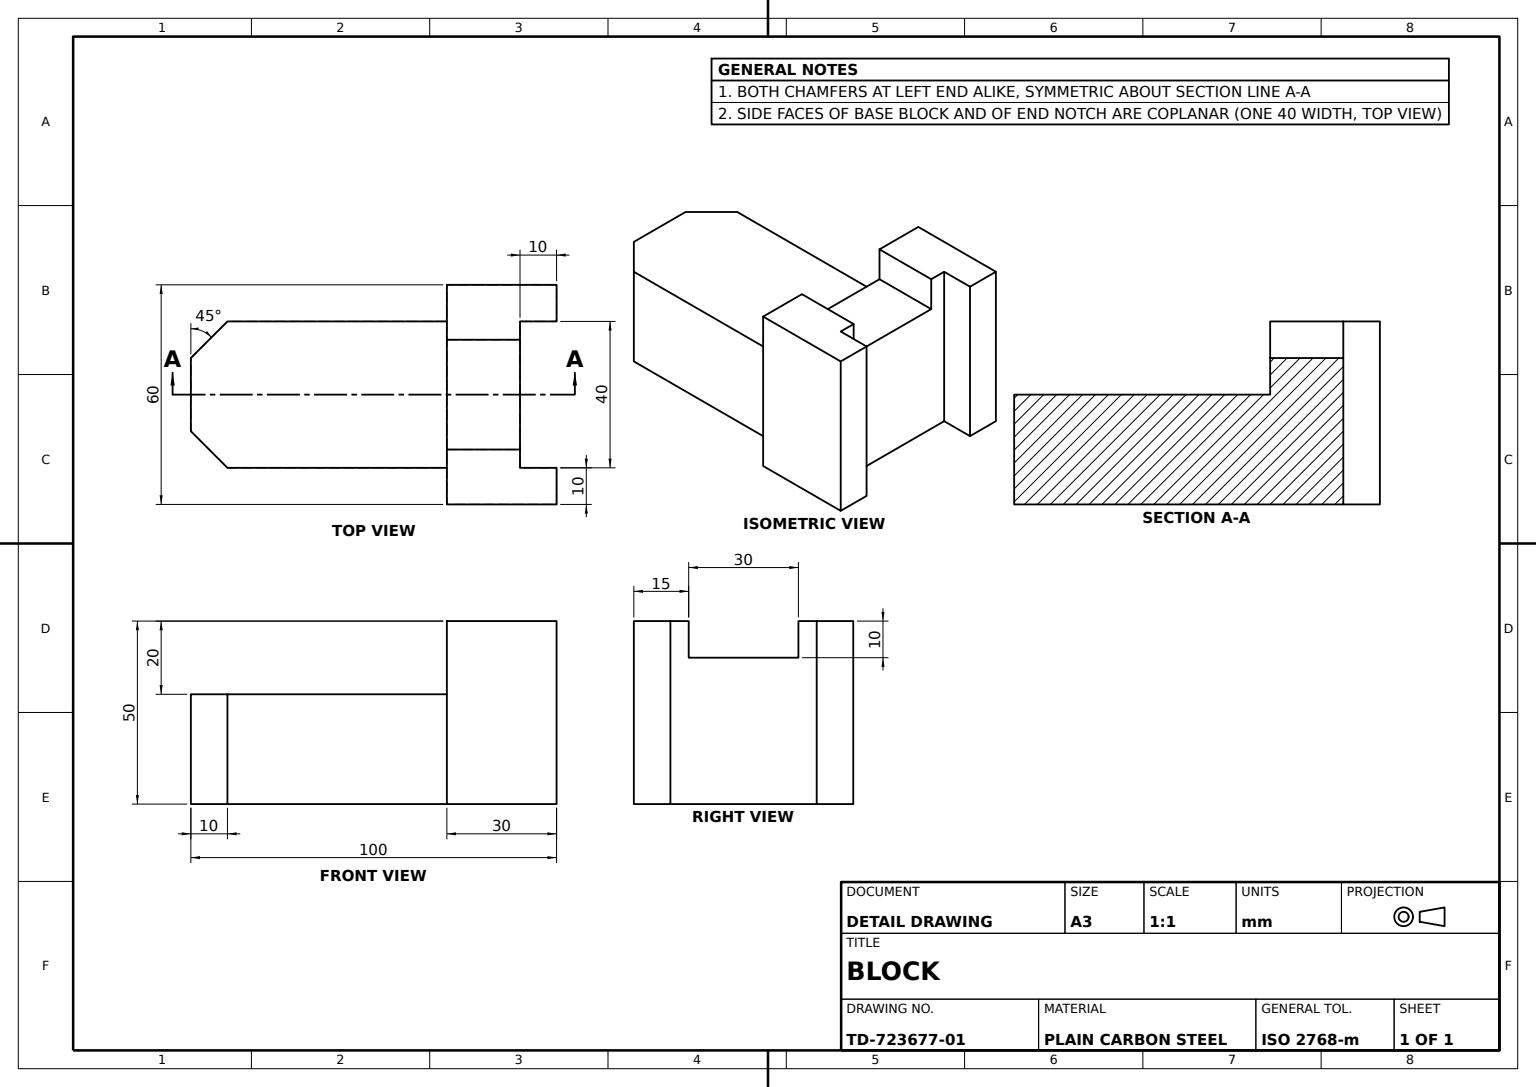
SolidWorks part; units mm, degrees
material "Plain Carbon Steel"
ref_plane "Front Plane" through (0, 0, 0) normal (0, 0, 1) x (1, 0, 0)
ref_plane "Top Plane" through (0, 0, 0) normal (0, 1, 0) x (1, 0, 0)
ref_plane "Right Plane" through (0, 0, 0) normal (1, 0, 0) x (0, 0, -1)
sketch "Base Profile Sketch" plane through (0, 0, 0) normal (0, 1, 0) x (1, 0, 0)
  line L0 (0, 30) -> (0, 0)
  line L1 (0, 0) -> (60, 0)
  line L2 (60, 0) -> (60, 30)
  line L3 (60, 30) -> (50, 30)
  line L4 (50, 30) -> (50, 20)
  line L5 (50, 20) -> (26.1605, 20)
  line L6 (26.1605, 20) -> (10, 20)
  line L7 (10, 20) -> (10, 30)
  line L8 (10, 30) -> (0, 30)
  dimension "D1" = 30
  dimension "D2" = 10
  dimension "D3" = 60
  dimension "D4" = 10
  dimension "D5" = 30
  dimension "D6" = 10
  dimension "D7" = 16.1605
extrude "Chamfered Base Block" add sketch "Base Profile Sketch" along normal blind 50
sketch "Step Cut Sketch" plane through (0, 50, 0) normal (0, 1, 0) x (1, 0, 0)
  line L0 (30, 0) -> (30, 31.3906) construction
  line L1 (0, 0) -> (60, 0) construction
  line L3 (45, -20) -> (15, -20)
  line L4 (45, -20) -> (45, 20)
  line L5 (45, 20) -> (15, 20)
  line L6 (15, -20) -> (15, 20)
  line L7 (45, -20) -> (15, 20) construction
  line L8 (45, 20) -> (15, -20) construction
  dimension "D1" = 30
  dimension "D2" = 40
extrude "Step Cut 30x40" cut sketch "Step Cut Sketch" against normal blind 10 contours L5 L6 L3 L4
sketch "Upright Profile Sketch" plane through (0, 0, 0) normal (0, -1, 0) x (1, 0, 0)
  line L0 (30, 0) -> (30, 84.9461) construction
  line L1 (0, 0) -> (60, 0) construction
  line L2 (60, -30) -> (50, -30) construction
  line L3 (10, 0) -> (50, 0)
  line L4 (10, 0) -> (10, 70)
  line L5 (10, 70) -> (50, 70)
  line L6 (50, 0) -> (50, 70)
  point P10 (30, 70)
  dimension "D1" = 100
  dimension "D2" = 40
extrude "Upright Block" add sketch "Upright Profile Sketch" against normal blind 30
sketch "Slot Sketch" plane through (0, 0, 0) normal (0, -1, 0) x (1, 0, 0)
  line L0 (50, 60) -> (40, 70)
  line L1 (50, 0) -> (50, 70) construction
  line L2 (50, 70) -> (10, 70) construction
  line L3 (40, 70) -> (50, 70)
  line L4 (50, 70) -> (50, 60)
  line L5 (30, 70) -> (30, 35.4952) construction
  line L6 (10, 70) -> (10, 60)
  line L7 (20, 70) -> (10, 70)
  line L8 (10, 60) -> (20, 70)
  dimension "D1" = 10
  dimension "D2" = 10
extrude "Top Slot Cut" cut sketch "Slot Sketch" against normal blind 30
